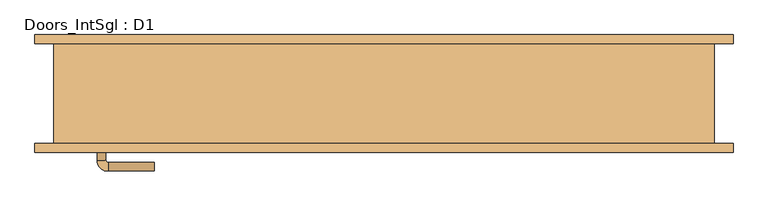
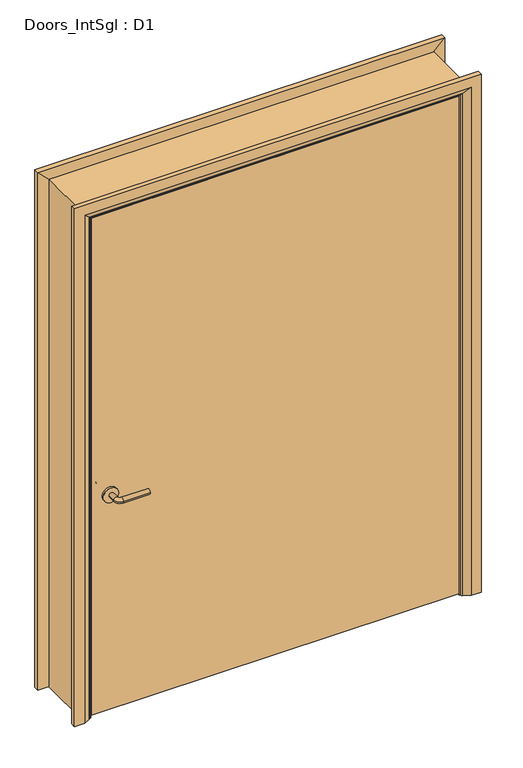
"""IFC4 building model written with IfcOpenShell, lengths in millimetres: door geometry, Doors_IntSgl : D1."""

from ifc_helpers import new_model, si_unit, point, frame, frame_2d, origin, place, context, project, spatial, polyline, circle_curve, ellipse_curve, trimmed, segment, composite_curve, outline, extrude, faceted_brep, source, transform, mapped, element, save
from ifc_brep_helpers import plane_surface, cylinder_surface, revolved_surface, advanced_brep


def doors_intsgl_d1_52b86bcf(model_context):
    return source(origin(), model_context, "Body", "SolidModel", [
        advanced_brep(
        [(-655.0, -68.3, 900.0), (-635.0, -68.3, 900.0), (-655.0, -38.3, 900.0), (-635.0, -38.3, 900.0), (-630.0, -33.3, 900.0), (-630.0, -13.3, 900.0), (-525.0, -13.3, 900.0), (-525.0, -33.3, 900.0)],
        [
            (0, 1, circle_curve(frame((-645.0, -68.3, 900.0), z_axis=(0.0, -1.0, 0.0), x_axis=(1.0, 0.0, 0.0)), 10.0)),
            (1, 0, circle_curve(frame((-645.0, -68.3, 900.0), z_axis=(0.0, -1.0, 0.0), x_axis=(1.0, 0.0, 0.0)), 10.0)),
            (0, 2),
            (2, 3, circle_curve(frame((-645.0, -38.3, 900.0), z_axis=(0.0, -1.0, 0.0), x_axis=(1.0, 0.0, 0.0)), 10.0)),
            (3, 1),
            (3, 2, circle_curve(frame((-645.0, -38.3, 900.0), z_axis=(0.0, -1.0, 0.0), x_axis=(1.0, 0.0, 0.0)), 10.0)),
            (4, 3, circle_curve(frame((-630.0, -38.3, 900.0), z_axis=(0.0, 0.0, 1.0), x_axis=(-1.0, 0.0, 0.0)), 5.0)),
            (2, 5, circle_curve(frame((-630.0, -38.3, 900.0), z_axis=(0.0, 0.0, -1.0), x_axis=(-1.0, 0.0, 0.0)), 25.0)),
            (5, 4, circle_curve(frame((-630.0, -23.3, 900.0), z_axis=(-1.0, 0.0, 0.0), x_axis=(0.0, -1.0, 0.0)), 10.0)),
            (4, 5, circle_curve(frame((-630.0, -23.3, 900.0), z_axis=(-1.0, 0.0, 0.0), x_axis=(0.0, -1.0, 0.0)), 10.0)),
            (6, 7, circle_curve(frame((-525.0, -23.3, 900.0), z_axis=(1.0, 0.0, 0.0), x_axis=(0.0, -1.0, 0.0)), 10.0)),
            (7, 6, circle_curve(frame((-525.0, -23.3, 900.0), z_axis=(1.0, 0.0, 0.0), x_axis=(0.0, -1.0, 0.0)), 10.0)),
            (5, 6),
            (7, 4),
        ],
        [
            plane_surface(frame((-645.0, -68.3, 900.0), z_axis=(0.0, -1.0, 0.0), x_axis=(0.0, 0.0, 1.0))),
            cylinder_surface(frame((-645.0, -68.3, 900.0), z_axis=(0.0, -1.0, 0.0), x_axis=(1.0, 0.0, 0.0)), 10.0),
            revolved_surface(trimmed(ellipse_curve(frame((-645.0, -38.3, 900.0), z_axis=(0.0, -1.0, 0.0), x_axis=(1.0, 0.0, 0.0)), 10.0, 10.0), [point((-655.0, -38.3, 900.0))], [point((-635.0, -38.3, 900.0))], True, "CARTESIAN"), (-630.0, -38.3, 900.0), (0.0, 0.0, -1.0)),
            revolved_surface(trimmed(ellipse_curve(frame((-645.0, -38.3, 900.0), z_axis=(0.0, -1.0, 0.0), x_axis=(1.0, 0.0, 0.0)), 10.0, 10.0), [point((-635.0, -38.3, 900.0))], [point((-655.0, -38.3, 900.0))], True, "CARTESIAN"), (-630.0, -38.3, 900.0), (0.0, 0.0, -1.0)),
            plane_surface(frame((-525.0, -23.3, 900.0), z_axis=(1.0, 0.0, 0.0), x_axis=(0.0, 0.0, 1.0))),
            cylinder_surface(frame((-630.0, -23.3, 900.0), z_axis=(-1.0, 0.0, 0.0), x_axis=(0.0, -1.0, 0.0)), 10.0),
        ],
        [
            (0, [[1, 2]]),
            (1, [[-1, 3, 4, 5]]),
            (1, [[-2, -5, 6, -3]]),
            (2, [[7, -4, 8, 9]]),
            (3, [[-8, -6, -7, 10]]),
            (4, [[11, 12]]),
            (5, [[-9, 13, -12, 14]]),
            (5, [[-10, -14, -11, -13]]),
        ],
    ),
        extrude(outline(composite_curve([segment(trimmed(circle_curve(frame_2d((900.0, -647.5)), 30.0), [point((900.0, -677.5))], [point((900.0, -617.5))], False, "CARTESIAN"), True, "CONTINUOUS"), segment(trimmed(circle_curve(frame_2d((900.0, -647.5)), 30.0), [point((900.0, -617.5))], [point((900.0, -677.5))], False, "CARTESIAN"), True, "CONTINUOUS")], self_intersect=False)), frame((0.0, -76.3, 0.0), z_axis=(0.0, 1.0, 0.0), x_axis=(0.0, 0.0, 1.0)), (0.0, 0.0, 1.0), 8.0),
        advanced_brep(
        [(-655.0, -122.3, 900.0), (-635.0, -122.3, 900.0), (-635.0, -152.3, 900.0), (-655.0, -152.3, 900.0), (-630.0, -157.3, 900.0), (-630.0, -177.3, 900.0), (-525.0, -177.3, 900.0), (-525.0, -157.3, 900.0)],
        [
            (0, 1, circle_curve(frame((-645.0, -122.3, 900.0), z_axis=(0.0, 1.0, 0.0), x_axis=(1.0, 0.0, 0.0)), 10.0)),
            (1, 0, circle_curve(frame((-645.0, -122.3, 900.0), z_axis=(0.0, 1.0, 0.0), x_axis=(1.0, 0.0, 0.0)), 10.0)),
            (1, 2),
            (2, 3, circle_curve(frame((-645.0, -152.3, 900.0), z_axis=(0.0, 1.0, 0.0), x_axis=(1.0, 0.0, 0.0)), 10.0)),
            (3, 0),
            (3, 2, circle_curve(frame((-645.0, -152.3, 900.0), z_axis=(0.0, 1.0, 0.0), x_axis=(1.0, 0.0, 0.0)), 10.0)),
            (4, 5, circle_curve(frame((-630.0, -167.3, 900.0), z_axis=(-1.0, 0.0, 0.0), x_axis=(0.0, 1.0, 0.0)), 10.0)),
            (5, 3, circle_curve(frame((-630.0, -152.3, 900.0), z_axis=(0.0, 0.0, -1.0), x_axis=(-1.0, 0.0, 0.0)), 25.0)),
            (2, 4, circle_curve(frame((-630.0, -152.3, 900.0), z_axis=(0.0, 0.0, 1.0), x_axis=(-1.0, 0.0, 0.0)), 5.0)),
            (5, 4, circle_curve(frame((-630.0, -167.3, 900.0), z_axis=(-1.0, 0.0, 0.0), x_axis=(0.0, 1.0, 0.0)), 10.0)),
            (6, 7, circle_curve(frame((-525.0, -167.3, 900.0), z_axis=(1.0, 0.0, 0.0), x_axis=(0.0, 1.0, 0.0)), 10.0)),
            (7, 6, circle_curve(frame((-525.0, -167.3, 900.0), z_axis=(1.0, 0.0, 0.0), x_axis=(0.0, 1.0, 0.0)), 10.0)),
            (4, 7),
            (6, 5),
        ],
        [
            plane_surface(frame((-645.0, -122.3, 900.0), z_axis=(0.0, 1.0, 0.0), x_axis=(0.0, 0.0, 1.0))),
            cylinder_surface(frame((-645.0, -122.3, 900.0), z_axis=(0.0, 1.0, 0.0), x_axis=(1.0, 0.0, 0.0)), 10.0),
            revolved_surface(trimmed(ellipse_curve(frame((-645.0, -152.3, 900.0), z_axis=(0.0, -1.0, 0.0), x_axis=(1.0, 0.0, 0.0)), 10.0, 10.0), [point((-655.0, -152.3, 900.0))], [point((-635.0, -152.3, 900.0))], True, "CARTESIAN"), (-630.0, -152.3, 900.0), (0.0, 0.0, -1.0)),
            revolved_surface(trimmed(ellipse_curve(frame((-645.0, -152.3, 900.0), z_axis=(0.0, -1.0, 0.0), x_axis=(1.0, 0.0, 0.0)), 10.0, 10.0), [point((-635.0, -152.3, 900.0))], [point((-655.0, -152.3, 900.0))], True, "CARTESIAN"), (-630.0, -152.3, 900.0), (0.0, 0.0, -1.0)),
            plane_surface(frame((-525.0, -167.3, 900.0), z_axis=(1.0, 0.0, 0.0), x_axis=(0.0, 0.0, 1.0))),
            cylinder_surface(frame((-630.0, -167.3, 900.0), z_axis=(-1.0, 0.0, 0.0), x_axis=(0.0, 1.0, 0.0)), 10.0),
        ],
        [
            (0, [[1, 2]]),
            (1, [[3, 4, 5, -2]]),
            (1, [[-5, 6, -3, -1]]),
            (2, [[7, 8, -4, 9]]),
            (3, [[10, -9, -6, -8]]),
            (4, [[11, 12]]),
            (5, [[13, -11, 14, -7]]),
            (5, [[-14, -12, -13, -10]]),
        ],
    ),
        extrude(outline(composite_curve([segment(trimmed(circle_curve(frame_2d((900.0, -647.5)), 30.0), [point((900.0, -677.5))], [point((900.0, -617.5))], False, "CARTESIAN"), True, "CONTINUOUS"), segment(trimmed(circle_curve(frame_2d((900.0, -647.5)), 30.0), [point((900.0, -617.5))], [point((900.0, -677.5))], False, "CARTESIAN"), True, "CONTINUOUS")], self_intersect=False)), frame((0.0, -122.3, 0.0), z_axis=(0.0, 1.0, 0.0), x_axis=(0.0, 0.0, 1.0)), (0.0, 0.0, 1.0), 8.0),
        extrude(outline(polyline([(720.0, -76.3), (720.0, -114.3), (-720.0, -114.3), (-720.0, -76.3), (720.0, -76.3)])), frame((0.0, 0.0, 8.0), z_axis=(0.0, 0.0, 1.0), x_axis=(1.0, 0.0, 0.0)), (0.0, 0.0, 1.0), 2060.0),
        advanced_brep(
        [(797.0, -134.3, 0.0), (757.0, -134.3, 0.0), (731.0, -120.3, 0.0), (727.0, -114.3, 0.0), (797.0, -114.3, 0.0), (797.0, -114.3, 2145.0), (797.0, -134.3, 2145.0), (727.0, -114.3, 2075.0), (-727.0, -114.3, 2075.0), (-727.0, -114.3, 0.0), (-797.0, -114.3, 0.0), (-797.0, -114.3, 2145.0), (731.0, -120.3, 2079.0), (757.0, -134.3, 2105.0), (-797.0, -134.3, 2145.0), (-797.0, -134.3, 0.0), (-757.0, -134.3, 0.0), (-757.0, -134.3, 2105.0), (-731.0, -120.3, 0.0), (-731.0, -120.3, 2079.0)],
        [
            (0, 1),
            (1, 2),
            (2, 3, circle_curve(frame((735.0, -113.3, 0.0), z_axis=(0.0, 0.0, -1.0), x_axis=(1.0, 0.0, 0.0)), 8.0622577)),
            (3, 4),
            (4, 0),
            (4, 5),
            (5, 6),
            (6, 0),
            (3, 7),
            (7, 8),
            (8, 9),
            (9, 10),
            (10, 11),
            (11, 5),
            (2, 12),
            (12, 7, ellipse_curve(frame((735.0, -113.3, 2083.0), z_axis=(0.7071067811865475, 0.0, -0.7071067811865475), x_axis=(-0.7071067811865474, 0.0, -0.7071067811865476)), 11.4017543, 8.0622577)),
            (1, 13),
            (13, 12),
            (6, 14),
            (14, 15),
            (15, 16),
            (16, 17),
            (17, 13),
            (10, 15),
            (14, 11),
            (9, 18, circle_curve(frame((-735.0, -113.3, 0.0), z_axis=(0.0, 0.0, -1.0), x_axis=(-1.0, 0.0, 0.0)), 8.0622577)),
            (18, 16),
            (19, 18),
            (8, 19, ellipse_curve(frame((-735.0, -113.3, 2083.0), z_axis=(-0.7071067811865475, 0.0, -0.7071067811865475), x_axis=(-0.7071067811865474, 0.0, 0.7071067811865476)), 11.4017543, 8.0622577)),
            (19, 17),
            (12, 19),
        ],
        [
            plane_surface(frame((727.0, -114.3, 0.0), z_axis=(0.0, 0.0, -1.0), x_axis=(0.0, 1.0, 0.0))),
            plane_surface(frame((797.0, -134.3, 0.0), z_axis=(1.0, 0.0, 0.0), x_axis=(0.0, 0.0, 1.0))),
            plane_surface(frame((797.0, -114.3, 0.0), z_axis=(0.0, 1.0, 0.0), x_axis=(0.0, 0.0, 1.0))),
            cylinder_surface(frame((735.0, -113.3, 0.0), z_axis=(0.0, 0.0, -1.0), x_axis=(1.0, 0.0, 0.0)), 8.0622577),
            plane_surface(frame((731.0, -120.3, 0.0), z_axis=(-0.4740998230350126, -0.880471099922178, 0.0), x_axis=(0.0, 0.0, 1.0))),
            plane_surface(frame((757.0, -134.3, 0.0), z_axis=(0.0, -1.0, 0.0), x_axis=(0.0, 0.0, 1.0))),
            plane_surface(frame((-797.0, -134.3, 2145.0), z_axis=(-1.0, 0.0, 0.0), x_axis=(0.0, 0.0, -1.0))),
            plane_surface(frame((-727.0, -114.3, 0.0), z_axis=(0.0, 0.0, -1.0), x_axis=(0.0, 1.0, 0.0))),
            cylinder_surface(frame((-735.0, -113.3, 2075.0), z_axis=(0.0, 0.0, 1.0), x_axis=(-1.0, 0.0, 0.0)), 8.0622577),
            plane_surface(frame((-731.0, -120.3, 2079.0), z_axis=(0.47409982303501824, -0.8804710999221749, 0.0), x_axis=(0.0, 0.0, -1.0))),
            plane_surface(frame((797.0, -134.3, 2145.0), z_axis=(0.0, 0.0, 1.0), x_axis=(-1.0, 0.0, 0.0))),
            cylinder_surface(frame((727.0, -113.3, 2083.0), z_axis=(1.0, 0.0, 0.0), x_axis=(0.0, 0.0, 1.0)), 8.0622577),
            plane_surface(frame((731.0, -120.3, 2079.0), z_axis=(0.0, -0.8804710999221764, -0.4740998230350154), x_axis=(-1.0, 0.0, 0.0))),
        ],
        [
            (0, [[1, 2, 3, 4, 5]]),
            (1, [[6, 7, 8, -5]]),
            (2, [[9, 10, 11, 12, 13, 14, -6, -4]]),
            (3, [[15, 16, -9, -3]]),
            (4, [[17, 18, -15, -2]]),
            (5, [[-8, 19, 20, 21, 22, 23, -17, -1]]),
            (6, [[-13, 24, -20, 25]]),
            (7, [[-24, -12, 26, 27, -21]]),
            (8, [[28, -26, -11, 29]]),
            (9, [[-22, -27, -28, 30]]),
            (10, [[-14, -25, -19, -7]]),
            (11, [[31, -29, -10, -16]]),
            (12, [[-23, -30, -31, -18]]),
        ],
    ),
        extrude(outline(polyline([(0.0, -703.0), (2051.0, -703.0), (2051.0, 703.0), (0.0, 703.0), (0.0, 722.0), (2070.0, 722.0), (2070.0, -722.0), (0.0, -722.0), (0.0, -703.0)])), frame((0.0, -74.3, 0.0), z_axis=(0.0, 1.0, 0.0), x_axis=(0.0, 0.0, 1.0)), (0.0, 0.0, 1.0), 32.0),
        advanced_brep(
        [(-797.0, 134.3, 0.0), (-757.0, 134.3, 0.0), (-731.0, 120.3, 0.0), (-727.0, 114.3, 0.0), (-797.0, 114.3, 0.0), (-797.0, 114.3, 2145.0), (-797.0, 134.3, 2145.0), (-727.0, 114.3, 2075.0), (-731.0, 120.3, 2079.0), (-757.0, 134.3, 2105.0), (797.0, 134.3, 0.0), (797.0, 114.3, 0.0), (727.0, 114.3, 0.0), (731.0, 120.3, 0.0), (757.0, 134.3, 0.0), (797.0, 134.3, 2145.0), (757.0, 134.3, 2105.0), (731.0, 120.3, 2079.0), (727.0, 114.3, 2075.0), (797.0, 114.3, 2145.0)],
        [
            (0, 1),
            (1, 2),
            (2, 3, circle_curve(frame((-735.0, 113.3, 0.0), z_axis=(0.0, 0.0, -1.0), x_axis=(-1.0, 0.0, 0.0)), 8.0622577)),
            (3, 4),
            (4, 0),
            (4, 5),
            (5, 6),
            (6, 0),
            (3, 7),
            (7, 5),
            (2, 8),
            (8, 7, ellipse_curve(frame((-735.0, 113.3, 2083.0), z_axis=(-0.7071067811865475, 0.0, -0.7071067811865475), x_axis=(0.7071067811865474, 0.0, -0.7071067811865476)), 11.4017543, 8.0622577)),
            (1, 9),
            (9, 8),
            (6, 9),
            (10, 11),
            (11, 12),
            (12, 13, circle_curve(frame((735.0, 113.3, 0.0), z_axis=(0.0, 0.0, -1.0), x_axis=(1.0, 0.0, 0.0)), 8.0622577)),
            (13, 14),
            (14, 10),
            (15, 10),
            (14, 16),
            (16, 15),
            (13, 17),
            (17, 16),
            (12, 18),
            (18, 17, ellipse_curve(frame((735.0, 113.3, 2083.0), z_axis=(0.7071067811865475, 0.0, -0.7071067811865475), x_axis=(0.7071067811865474, 0.0, 0.7071067811865476)), 11.4017543, 8.0622577)),
            (11, 19),
            (19, 18),
            (15, 19),
            (5, 19),
            (15, 6),
            (7, 18),
            (8, 17),
            (9, 16),
        ],
        [
            plane_surface(frame((-727.0, 187.1010989, 0.0), z_axis=(0.0, 0.0, -1.0), x_axis=(1.0, 0.0, 0.0))),
            plane_surface(frame((-797.0, 134.3, 0.0), z_axis=(-1.0, 0.0, 0.0), x_axis=(0.0, 0.0, 1.0))),
            plane_surface(frame((-797.0, 114.3, 0.0), z_axis=(0.0, -1.0, 0.0), x_axis=(0.0, 0.0, 1.0))),
            cylinder_surface(frame((-735.0, 113.3, 0.0), z_axis=(0.0, 0.0, -1.0), x_axis=(-1.0, 0.0, 0.0)), 8.0622577),
            plane_surface(frame((-731.0, 120.3, 0.0), z_axis=(0.4740998230350183, 0.8804710999221749, 0.0), x_axis=(0.0, 0.0, 1.0))),
            plane_surface(frame((-757.0, 134.3, 0.0), z_axis=(0.0, 1.0, 0.0), x_axis=(0.0, 0.0, 1.0))),
            plane_surface(frame((727.0, 187.1010989, 0.0), z_axis=(0.0, 0.0, -1.0), x_axis=(-1.0, 0.0, 0.0))),
            plane_surface(frame((757.0, 134.3, 2105.0), z_axis=(0.0, 1.0, 0.0), x_axis=(0.0, 0.0, -1.0))),
            plane_surface(frame((731.0, 120.3, 2079.0), z_axis=(-0.4740998230350183, 0.8804710999221749, 0.0), x_axis=(0.0, 0.0, -1.0))),
            cylinder_surface(frame((735.0, 113.3, 2075.0), z_axis=(0.0, 0.0, 1.0), x_axis=(1.0, 0.0, 0.0)), 8.0622577),
            plane_surface(frame((797.0, 114.3, 2145.0), z_axis=(0.0, -1.0, 0.0), x_axis=(0.0, 0.0, -1.0))),
            plane_surface(frame((797.0, 134.3, 2145.0), z_axis=(1.0, 0.0, 0.0), x_axis=(0.0, 0.0, -1.0))),
            plane_surface(frame((-797.0, 134.3, 2145.0), z_axis=(0.0, 0.0, 1.0), x_axis=(1.0, 0.0, 0.0))),
            plane_surface(frame((-797.0, 114.3, 2145.0), z_axis=(0.0, -1.0, 0.0), x_axis=(1.0, 0.0, 0.0))),
            cylinder_surface(frame((-727.0, 113.3, 2083.0), z_axis=(-1.0, 0.0, 0.0), x_axis=(0.0, 0.0, 1.0)), 8.0622577),
            plane_surface(frame((-731.0, 120.3, 2079.0), z_axis=(0.0, 0.8804710999221749, -0.4740998230350183), x_axis=(1.0, 0.0, 0.0))),
            plane_surface(frame((-757.0, 134.3, 2105.0), z_axis=(0.0, 1.0, 0.0), x_axis=(1.0, 0.0, 0.0))),
        ],
        [
            (0, [[1, 2, 3, 4, 5]]),
            (1, [[6, 7, 8, -5]]),
            (2, [[9, 10, -6, -4]]),
            (3, [[11, 12, -9, -3]]),
            (4, [[13, 14, -11, -2]]),
            (5, [[-8, 15, -13, -1]]),
            (6, [[16, 17, 18, 19, 20]]),
            (7, [[21, -20, 22, 23]]),
            (8, [[-22, -19, 24, 25]]),
            (9, [[-24, -18, 26, 27]]),
            (10, [[-26, -17, 28, 29]]),
            (11, [[-28, -16, -21, 30]]),
            (12, [[31, -30, 32, -7]]),
            (13, [[33, -29, -31, -10]]),
            (14, [[34, -27, -33, -12]]),
            (15, [[35, -25, -34, -14]]),
            (16, [[-32, -23, -35, -15]]),
        ],
    ),
        faceted_brep([(-722.0, -114.3, 0.0), (-754.0, -114.3, 0.0), (-754.0, 114.3, 0.0), (-722.0, 114.3, 0.0), (-722.0, 114.3, 2070.0), (-722.0, -114.3, 2070.0), (-754.0, 114.3, 2102.0), (-754.0, -114.3, 2102.0), (722.0, -114.3, 0.0), (722.0, 114.3, 0.0), (754.0, 114.3, 0.0), (754.0, -114.3, 0.0), (722.0, -114.3, 2070.0), (754.0, -114.3, 2102.0), (754.0, 114.3, 2102.0), (722.0, 114.3, 2070.0)], [[[0, 1, 2, 3]], [[3, 4, 5, 0]], [[2, 6, 4, 3]], [[1, 7, 6, 2]], [[0, 5, 7, 1]], [[8, 9, 10, 11]], [[12, 8, 11, 13]], [[13, 11, 10, 14]], [[14, 10, 9, 15]], [[15, 9, 8, 12]], [[4, 15, 12, 5]], [[6, 14, 15, 4]], [[7, 13, 14, 6]], [[5, 12, 13, 7]]]),
    ])


if __name__ == "__main__":
    model = new_model("IFC4")
    model_context = context("Model", 3, world=origin())
    ifc_project = project(units=[si_unit("LENGTHUNIT", "METRE", prefix="MILLI")], contexts=[model_context])
    site = spatial("IfcSite", under=ifc_project)
    building = spatial("IfcBuilding", under=site)
    placement = place(None, origin())
    doors_intsgl_d1_shape = doors_intsgl_d1_52b86bcf(model_context)
    element("IfcDoor", 1, ObjectType="Doors_IntSgl : D1", at=placement, inside=building, context=model_context, shape_type="MappedRepresentation", body=[
        mapped(doors_intsgl_d1_shape, transform((0.0, 0.0, 0.0), x_axis=(1.0, 0.0, 0.0), y_axis=(0.0, 1.0, 0.0), z_axis=(0.0, 0.0, 1.0))),
    ])
    save(model, "model.ifc")

# Revit data of these elements
# Type "Doors_IntSgl : D1"
#   Type Mark = "46"
#   Type Comments = "Internal Single"
#   Operation = "SingleSwingRight"
#   Manufacturer = "Revit"
#   Keynote = "L20"
#   Description = "Internal Single Door"
#   Analytic Construction = "Metal"
#   UnderCut = 8 mm
#   Tolerance = 2 mm
#   Thickness = 38 mm
#   Thermal Resistance (R) = 0.270117 (m²·K)/W
#   Structural Tolerance = 8 mm
#   StopDepth = 32 mm
#   Stop Thickness = 19 mm
#   Rough Width = 1524 mm
#   Rough Height = 2110 mm
#   Height to Top Lock Rail = 1000 mm
#   Heat Transfer Coefficient (U) = 3.7021 W/(m²·K)
#   Handle Z Distance = 900 mm
#   Handle X Distance = 75 mm
#   Frame Thickness = 32 mm
#   Door Panel Width = 1440 mm
#   Door Panel Thickness = 38 mm
#   Door Panel Offset = 0 mm
#   Height = 2110 mm
#   Width = 1524 mm
#   Door Panel Height = 2060 mm
#   Architrave Setback = 5 mm
#   Vis - Ironmongery = yes
#   Material Ironmongery = Door - Handle
#   Material Frame = Door - Frame/Mullion (1)
#   Material Door = Door - Panel
#   Material Architrave = Door - Architrave
#   Visual Light Transmittance = 0
#   Solar Heat Gain Coefficient = 0
#   Function = (empty or 0)
#   Wall Closure = (empty or 0)
# Element 1 (IfcDoor, "Doors_IntSgl : D1")
#   Materials on its faces: "Door - Architrave", "Door - Handle", "Door - Frame/Mullion (1)", "Door - Panel"
# Materials
#   "Door - Handle": colour RGB 0 0 0, transparency 0, Keynote = "P21", Cost = 0
#   "Door - Frame/Mullion (1)": class "Wood", colour RGB 212 179 113, transparency 0, Keynote = "L20", Cost = 0
#   "Door - Panel": class "Wood", colour RGB 210 159 95, transparency 0, Keynote = "L20", Cost = 0
#   "Door - Architrave": class "Wood", colour RGB 154 90 5, transparency 0, Keynote = "P20", Cost = 0
